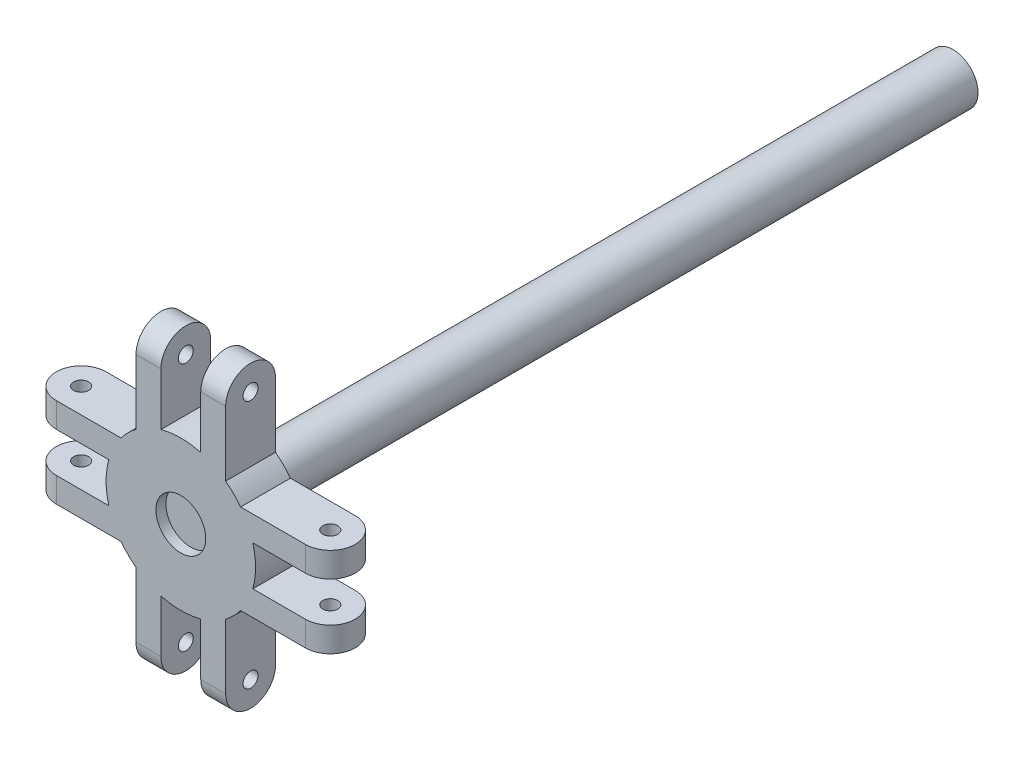
from build123d import *

# Parameters (mm, degrees)
CROSS_FLANGE_DEPTH        = 5
SKETCH1_3_R               = 5
SHAFT_150_DEPTH           = 150
ARM_HOLES_A_SKETCH_R      = 1.5
ARM_HOLES_A_DEPTH         = 158.863865403
ARM_HOLES_B_SKETCH_R      = 1.5
ARM_HOLES_B_DEPTH         = 158.863865403
CENTER_RECESS_10_SKETCH_R = 5
CENTER_RECESS_10_X2_DEPTH = 2


with BuildPart() as part:
    # Cross Flange Profile → Cross Flange (new, symmetric)
    with BuildSketch(Plane.XY):
        with BuildLine():
            Line((-4, 14.456832295), (-4, 30))
            Line((-4, 30), (-9, 30))
            Line((-9, 30), (-9, 12))
            ThreePointArc((-9, 12), (-10.606601718, 10.606601718), (-12, 9))
            Line((-12, 9), (-30, 9))
            Line((-30, 9), (-30, 4))
            Line((-30, 4), (-14.456832295, 4))
            ThreePointArc((-14.456832295, 4), (-15, 0), (-14.456832295, -4))
            Line((-14.456832295, -4), (-30, -4))
            Line((-30, -4), (-30, -9))
            Line((-30, -9), (-12, -9))
            ThreePointArc((-12, -9), (-10.606601718, -10.606601718), (-9, -12))
            Line((-9, -12), (-9, -30))
            Line((-9, -30), (-4, -30))
            Line((-4, -30), (-4, -14.456832295))
            ThreePointArc((-4, -14.456832295), (0, -15), (4, -14.456832295))
            Line((4, -14.456832295), (4, -30))
            Line((4, -30), (9, -30))
            Line((9, -30), (9, -12))
            ThreePointArc((9, -12), (10.606601718, -10.606601718), (12, -9))
            Line((12, -9), (30, -9))
            Line((30, -9), (30, -4))
            Line((30, -4), (14.456832295, -4))
            ThreePointArc((14.456832295, -4), (15, 0), (14.456832295, 4))
            Line((14.456832295, 4), (30, 4))
            Line((30, 4), (30, 9))
            Line((30, 9), (12, 9))
            ThreePointArc((12, 9), (10.606601718, 10.606601718), (9, 12))
            Line((9, 12), (9, 30))
            Line((9, 30), (4, 30))
            Line((4, 30), (4, 14.456832295))
            ThreePointArc((4, 14.456832295), (0, 15), (-4, 14.456832295))
        make_face()
    extrude(amount=CROSS_FLANGE_DEPTH, both=True)

    # Sketch1_3 → Shaft 150 (add)
    with BuildSketch(Plane.XY):
        Circle(SKETCH1_3_R)
    extrude(amount=-SHAFT_150_DEPTH)

    # Arm Holes A Sketch → Arm Holes A (cut, through all)
    with BuildSketch(Plane(origin=(9, 0, 0), x_dir=(0, 0, -1), z_dir=(1, 0, 0))):
        with BuildLine():
            ThreePointArc((0, -30), (-3.535533906, -28.535533906), (-5, -25))
            Line((-5, -25), (-5, -30))
            Line((-5, -30), (0, -30))
        make_face()
        with BuildLine():
            ThreePointArc((5, -25), (3.535533906, -28.535533906), (0, -30))
            Line((0, -30), (5, -30))
            Line((5, -30), (5, -25))
        make_face()
        with BuildLine():
            Line((-5, 30), (-5, 25))
            ThreePointArc((-5, 25), (-3.535533906, 28.535533906), (0, 30))
            Line((0, 30), (-5, 30))
        make_face()
        with BuildLine():
            Line((5, 30), (0, 30))
            ThreePointArc((0, 30), (3.535533906, 28.535533906), (5, 25))
            Line((5, 25), (5, 30))
        make_face()
        with Locations(Location((0, 25, 0), (0, 0, 90))):
            Circle(ARM_HOLES_A_SKETCH_R)
        with Locations(Location((0, -25, 0), (0, 0, 90))):
            Circle(ARM_HOLES_A_SKETCH_R)
    extrude(amount=-ARM_HOLES_A_DEPTH, mode=Mode.SUBTRACT)

    # Arm Holes B Sketch → Arm Holes B (cut, through all)
    with BuildSketch(Plane(origin=(0, 9, 0), x_dir=(1, 0, 0), z_dir=(0, 1, 0))):
        with BuildLine():
            ThreePointArc((30, 0), (28.535533906, -3.535533906), (25, -5))
            Line((25, -5), (30, -5))
            Line((30, -5), (30, 0))
        make_face()
        with BuildLine():
            ThreePointArc((25, 5), (28.535533906, 3.535533906), (30, 0))
            Line((30, 0), (30, 5))
            Line((30, 5), (25, 5))
        make_face()
        with BuildLine():
            Line((-30, -5), (-25, -5))
            ThreePointArc((-25, -5), (-28.535533906, -3.535533906), (-30, 0))
            Line((-30, 0), (-30, -5))
        make_face()
        with BuildLine():
            Line((-30, 5), (-30, 0))
            ThreePointArc((-30, 0), (-28.535533906, 3.535533906), (-25, 5))
            Line((-25, 5), (-30, 5))
        make_face()
        with Locations(Location((-25, 0, 0), (0, 0, 180))):
            Circle(ARM_HOLES_B_SKETCH_R)
        with Locations((25, 0)):
            Circle(ARM_HOLES_B_SKETCH_R)
    extrude(amount=-ARM_HOLES_B_DEPTH, mode=Mode.SUBTRACT)

    # Center Recess _10 Sketch → Center Recess _10 x2 (cut)
    with BuildSketch(Plane.XY.offset(5)):
        Circle(CENTER_RECESS_10_SKETCH_R)
    extrude(amount=-CENTER_RECESS_10_X2_DEPTH, mode=Mode.SUBTRACT)


solid = part.part
